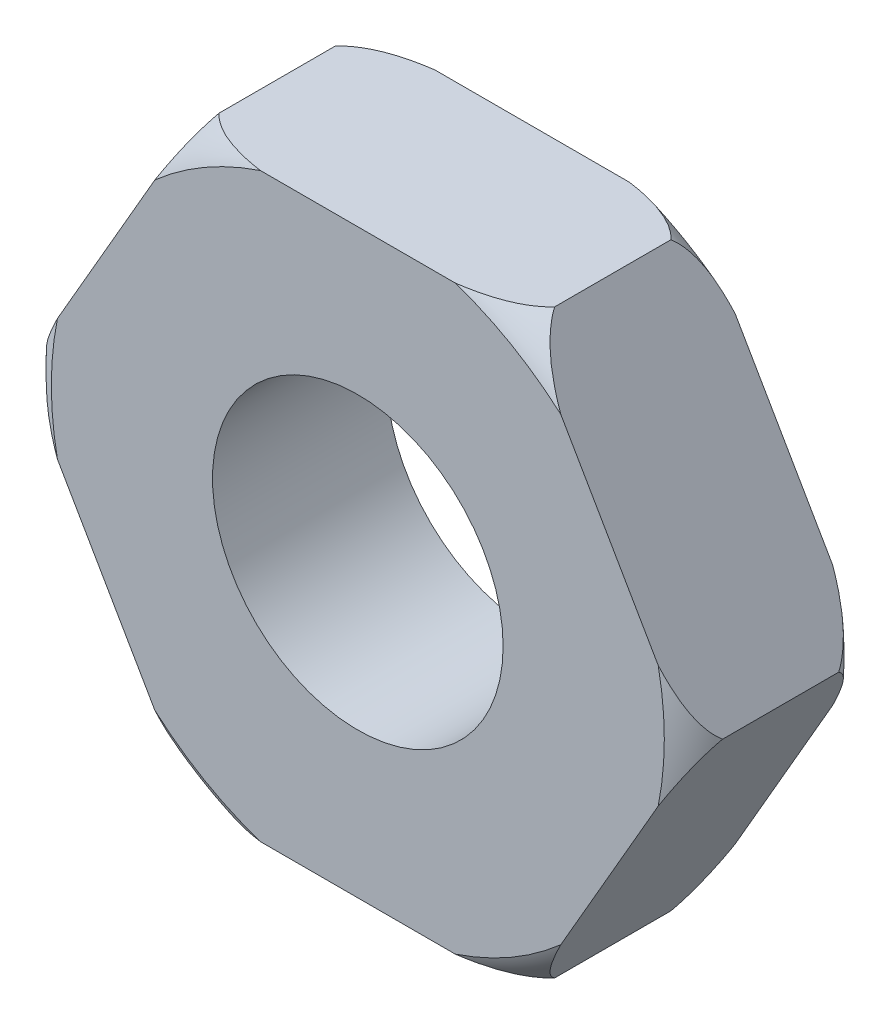
from build123d import *

# Parameters (mm, degrees)
HEX_PROFILE_20AF_R     = 5
HEX_NUT_BODY_6MM_DEPTH = 3


with BuildPart() as part:
    # Hex Profile 20AF → Hex Nut Body 6mm (new, symmetric)
    with BuildSketch(Plane.XY):
        Polygon((11.547005384, 0), (5.773502692, 10), (-5.773502692, 10), (-11.547005384, 0), (-5.773502692, -10), (5.773502692, -10), align=None)
        Circle(HEX_PROFILE_20AF_R, mode=Mode.SUBTRACT)
    extrude(amount=HEX_NUT_BODY_6MM_DEPTH, both=True)

    # Edge Chamfer Profile → Edge Chamfer Cut (revolve, cut)
    with BuildSketch(Plane(origin=(0, 0, 0), x_dir=(1, 0, 0), z_dir=(0, 1, 0))):
        with BuildLine():
            Line((10.547005384, 3), (11.547005384, 3))
            Line((11.547005384, 3), (11.547005384, 2))
            ThreePointArc((11.547005384, 2), (11.138343291, 2.591337907), (10.547005384, 3))
        make_face()
    edge_chamfer_cut = revolve(axis=Axis((0, 0, -5.076869621), (0, 0, 1)), mode=Mode.SUBTRACT)

    # Edge Chamfer Mirror: Edge Chamfer Cut across plane
    add(edge_chamfer_cut.mirror(Plane.XY), mode=Mode.SUBTRACT)


solid = part.part
